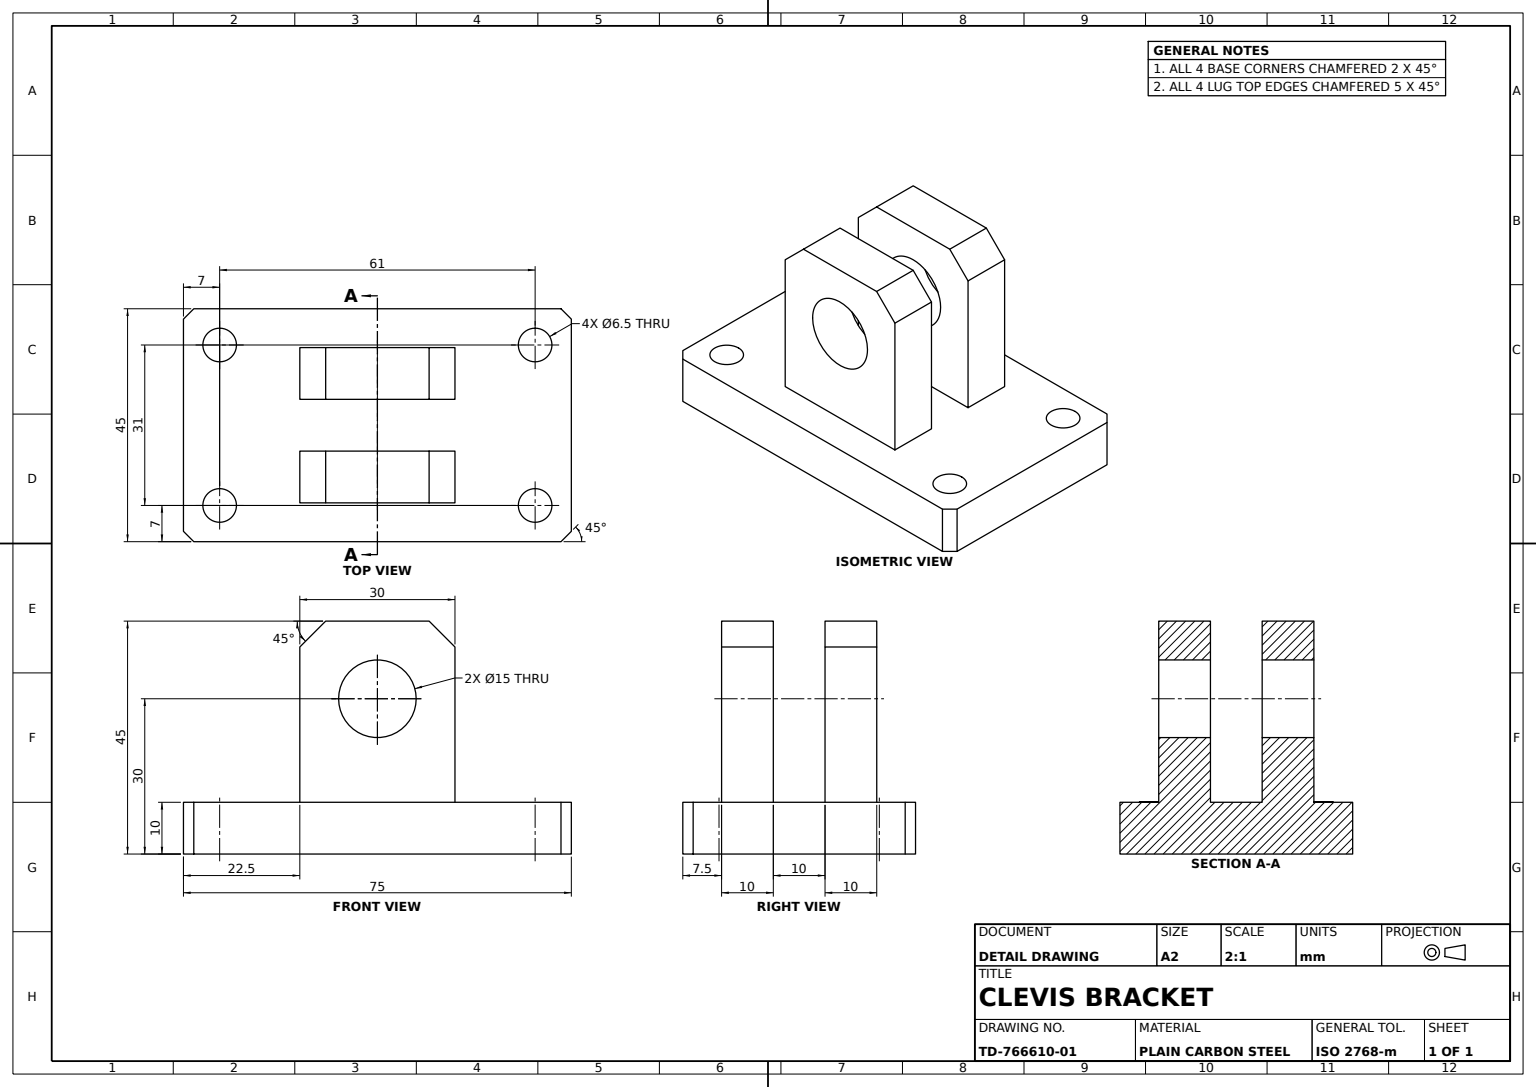
SolidWorks part; units mm, degrees
material "Plain Carbon Steel"
ref_plane "Front Plane" through (0, 0, 0) normal (0, 0, 1) x (1, 0, 0)
ref_plane "Top Plane" through (0, 0, 0) normal (0, 1, 0) x (1, 0, 0)
ref_plane "Right Plane" through (0, 0, 0) normal (1, 0, 0) x (0, 0, -1)
sketch "Base Plate Sketch" plane through (0, 0, 0) normal (0, 1, 0) x (1, 0, 0)
  line L1 (-37.5, -22.5) -> (37.5, -22.5)
  line L2 (-37.5, -22.5) -> (-37.5, 22.5)
  line L3 (-37.5, 22.5) -> (37.5, 22.5)
  line L4 (37.5, -22.5) -> (37.5, 22.5)
  line L5 (-37.5, -22.5) -> (37.5, 22.5) construction
  line L6 (-37.5, 22.5) -> (37.5, -22.5) construction
  point P0 (0, 0)
  dimension "D1" = 45
  dimension "D2" = 75
extrude "Base Plate 75x45x10" add sketch "Base Plate Sketch" along normal blind 10
chamfer "Base Corner Chamfer 1" distance 2 angle 45 1 edges at (37.5, 5, 22.5)
chamfer "Base Corner Chamfer 2" distance 2 angle 45 1 edges at (-37.5, 5, 22.5)
chamfer "Base Corner Chamfer 3" distance 2 angle 45 1 edges at (-37.5, 5, -22.5)
chamfer "Base Corner Chamfer 4" distance 2 angle 45 1 edges at (37.5, 5, -22.5)
ref_plane "Plane2" through (0, 0, 5) normal (0, 0, 1) x (1, 0, 0)
sketch "Fork Body Sketch" plane through (0, 0, 5) normal (0, 0, 1) x (1, 0, 0)
  line L0 (-15, 10) -> (15, 10)
  line L1 (-35.5, 10) -> (35.5, 10) construction
  line L2 (-15, 10) -> (-15, 45)
  line L3 (-15, 45) -> (15, 45)
  line L4 (15, 45) -> (15, 10)
  circle A0 centre (0, 30) radius 7.5
  point P5 (0, 10)
  dimension "D1" = 30
  dimension "D4" = 15
  dimension "D2" = 45
  dimension "D3" = 15
  dimension "D5" = 15
extrude "Fork Body" add sketch "Fork Body Sketch" along normal blind 10
sketch "Fork Extension Sketch" plane through (0, 0, -22.5) normal (0, 0, -1) x (-1, 0, 0)
  line L0 (-15, 10) -> (-15, 45)
  line L1 (-15, 45) -> (15, 45)
  line L2 (15, 45) -> (15, 10)
  line L3 (15, 10) -> (-15, 10)
  circle A0 centre (0, 30) radius 7.5
  dimension "D1" = 15
extrude "Fork Extension" add sketch "Fork Extension Sketch" against normal blind 17.5
sketch "Fork Slot Sketch" plane through (0, 0, -22.5) normal (0, 0, -1) x (-1, 0, 0)
  line L0 (-15, 10) -> (-15, 45)
  line L1 (-15, 45) -> (15, 45)
  line L2 (15, 45) -> (-15, 45) construction
  line L3 (15, 45) -> (15, 10)
  line L4 (15, 10) -> (-15, 10)
  circle A0 centre (0, 30) radius 7.5
  dimension "D1" = 15
extrude "Fork Slot" cut sketch "Fork Slot Sketch" against normal blind 7.5
chamfer "Fork Top Chamfer 1" distance 5 angle 45 1 edges at (-15, 45, -10)
chamfer "Fork Top Chamfer 2" distance 5 angle 45 3 edges at (-15, 45, 10) (15, 45, 10) (15, 45, -10)
sketch "Mounting Holes Sketch" plane through (0, 10, 0) normal (0, 1, 0) x (1, 0, 0)
  line L0 (0, 15.5) -> (0, -15.5) construction
  line L5 (-30.5, -15.5) -> (30.5, 15.5) construction
  line L6 (-30.5, 15.5) -> (30.5, -15.5) construction
  circle A0 centre (-30.5, 15.5) radius 3.25
  circle A1 centre (-30.5, -15.5) radius 3.25
  circle A2 centre (30.5, -15.5) radius 3.25
  circle A3 centre (30.5, 15.5) radius 3.25
  point P0 (0, 0)
  dimension "D1" = 6.5
  dimension "D2" = 6.5
  dimension "D3" = 61
  dimension "D4" = 31
  dimension "D5" = 15.5
extrude "Mounting Holes" cut sketch "Mounting Holes Sketch" against normal through all
